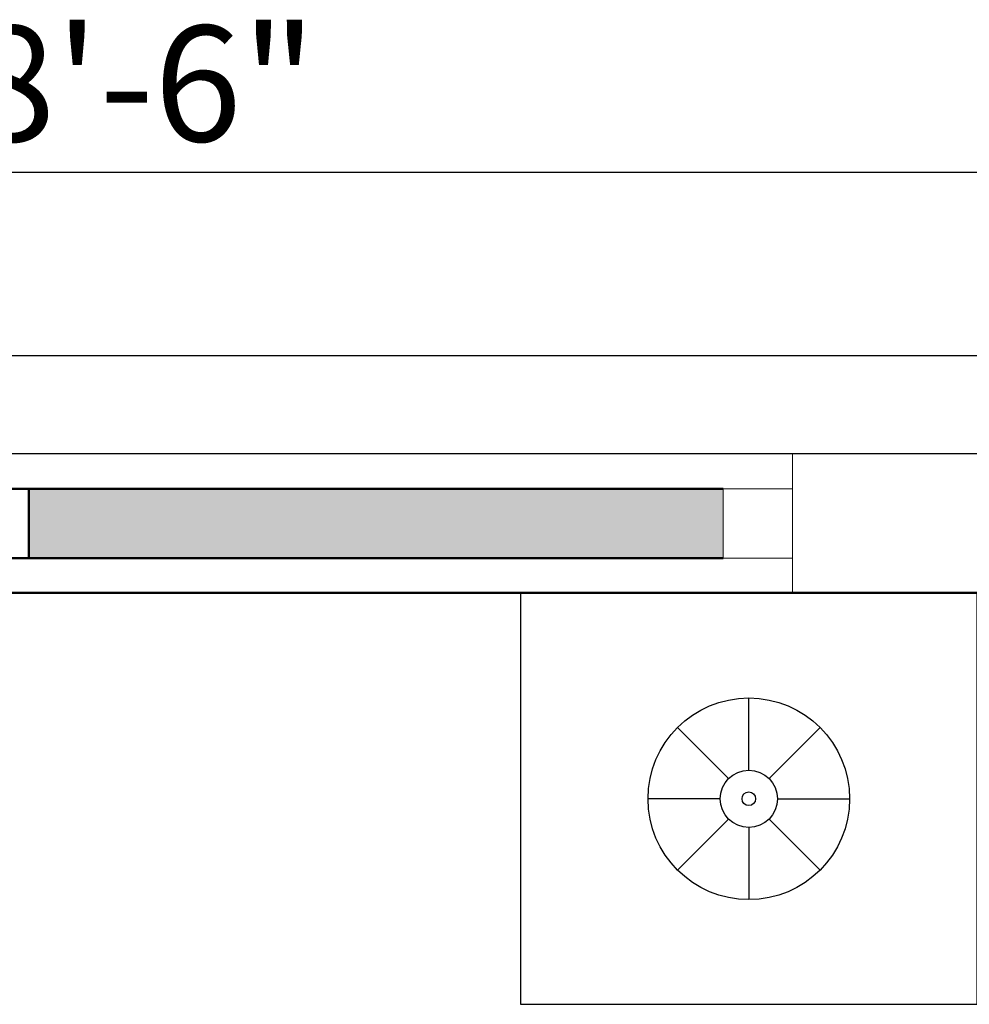
# Model space of a CAD drawing. Units: inches. Extents: x 3064 to 19385, y 846 to 15425.
# Tile 60 of 108: x 6210 to 6251, y 1964 to 2007. Entities that reach past the tile are written whole.
import ezdxf

# ---------------------------------------------------------------- set-up
doc = ezdxf.new("R2010")
doc.units = ezdxf.units.IN
for name, color, linetype, lineweight in [('A-ANNO-DIMS', 2, 'Continuous', 18), ('A-FLOR-FIXT', 9, 'Continuous', 18), ('A-GLAZ', 4, 'Continuous', 18), ('A-WALL', 7, 'Continuous', 50), ('C-PROP', 6, 'Continuous', 25)]:
    doc.layers.add(name, color=color, linetype=linetype, lineweight=lineweight)
doc.layers.add('BLOCK', color=6, linetype='Continuous')
doc.styles.get("Standard").update_dxf_attribs({"font": 'arial.ttf'})
doc.dimstyles.new('ISO-25', dxfattribs={"dimtxt": 9, "dimasz": 2.5, "dimexe": 1.25, "dimexo": 0.625, "dimtad": 1, "dimdec": 1, "dimlunit": 3, "dimtxsty": 'Standard', "dimcen": 2.5, "dimadec": 0, "dimazin": 0, "dimtfac": 1, "dimtdec": 1, "dimtmove": 0, "dimatfit": 3, "dimfxl": 1, "dimarcsym": 0})

# ---------------------------------------------------------------- blocks, each defined once
blk = doc.blocks.new('A$C52E67D0D')
at = {"layer": 'BLOCK'}
for p, q in [((250.5, 1605.5), (250.5, 1684.7)), ((228.3, 1596.3), (172.3, 1652.3)), ((272.7, 1596.3), (328.7, 1652.3)), ((219.1, 1574.1), (139.9, 1574.1)), ((281.9, 1574.1), (361.1, 1574.1)), ((228.3, 1551.9), (172.3, 1495.9)), ((272.7, 1551.9), (328.7, 1495.9)), ((250.5, 1542.8), (250.5, 1463.5))]:
    blk.add_line(p, q, dxfattribs=at)
blk.add_lwpolyline([(501, 1348.6), (501, 1799.6), (0, 1799.6), (0, 1348.6)], close=True, dxfattribs=at)
for radius in [110.6, 31.4, 7.46]:
    blk.add_circle((250.5, 1574.1), radius, dxfattribs=at)
blk = doc.blocks.new('*D387')
at = {"layer": 'A-ANNO-DIMS', "color": 0, "lineweight": -2, "transparency": 16777216}
for p, q in [((6183.493, 1988.614), (6183.493, 1993.494)), ((6378.493, 1988.614), (6378.493, 1993.494)), ((6185.993, 1992.244), (6375.993, 1992.244))]:
    blk.add_line(p, q, dxfattribs=at)
at = {"layer": 'A-ANNO-DIMS', "color": 0, "transparency": 16777216}
for points in [[(6185.993, 1992.66), (6185.993, 1991.827), (6183.493, 1992.244)], [(6375.993, 1992.66), (6375.993, 1991.827), (6378.493, 1992.244)]]:
    blk.add_solid(points, dxfattribs=at)
at = {"layer": 'Defpoints', "color": 0, "transparency": 16777216}
for p in [(6378.493, 1992.244), (6183.493, 1987.989), (6378.493, 1987.989)]:
    blk.add_point(p, dxfattribs=at)
at = {"layer": 'A-ANNO-DIMS', "color": 0, "transparency": 16777216, "insert": (6280.993, 1995.423), "char_height": 5, "attachment_point": 5}
blk.add_mtext('16\'-3"', dxfattribs=at)
blk = doc.blocks.new('*D378')
at = {"layer": 'A-ANNO-DIMS', "color": 0, "lineweight": -2, "transparency": 16777216}
for p, q in [((6042.493, 1988.614), (6042.493, 2001.412)), ((6384.493, 1988.614), (6384.493, 2001.412)), ((6044.993, 2000.162), (6381.993, 2000.162))]:
    blk.add_line(p, q, dxfattribs=at)
at = {"layer": 'A-ANNO-DIMS', "color": 0, "transparency": 16777216}
for points in [[(6044.993, 2000.578), (6044.993, 1999.745), (6042.493, 2000.162)], [(6381.993, 2000.578), (6381.993, 1999.745), (6384.493, 2000.162)]]:
    blk.add_solid(points, dxfattribs=at)
at = {"layer": 'Defpoints', "color": 0, "transparency": 16777216}
for p in [(6384.493, 2000.162), (6042.493, 1987.989), (6384.493, 1987.989)]:
    blk.add_point(p, dxfattribs=at)
at = {"layer": 'A-ANNO-DIMS', "color": 0, "transparency": 16777216, "insert": (6213.493, 2003.34), "char_height": 5, "attachment_point": 5}
blk.add_mtext('28\'-6"', dxfattribs=at)

msp = doc.modelspace()

# ---------------------------------------------------------------- hatches: boundary and pattern name
at = {"layer": 'A-GLAZ'}
h = msp.add_hatch(color=256, dxfattribs=at)
h.dxf.hatch_style = 1
h.paths.add_polyline_path([(6240.493, 1986.489), (6210.493, 1986.489), (6210.493, 1983.489), (6240.493, 1983.489)])

# ---------------------------------------------------------------- linework, layer by layer
msp.add_line((6243.493, 1987.989), (6243.493, 1981.989), dxfattribs=at)
msp.add_lwpolyline([(6243.493, 1983.489), (6240.493, 1983.489), (6240.493, 1986.489), (6243.493, 1986.489)], close=True, dxfattribs=at)
at = {"layer": 'A-WALL'}
for p, q in [((6210.493, 1986.489), (6240.493, 1986.489)), ((6210.493, 1983.489), (6240.493, 1983.489)), ((6378.493, 1981.989), (6183.493, 1981.989))]:
    msp.add_line(p, q, dxfattribs=at)
msp.add_lwpolyline([(6210.493, 1983.489), (6207.493, 1983.489), (6207.493, 1986.489), (6210.493, 1986.489)], close=True, dxfattribs=at)
at = {"layer": 'C-PROP'}
msp.add_line((6384.493, 1987.989), (6042.493, 1987.989), dxfattribs=at)

# ---------------------------------------------------------------- block references
at = {"layer": 'A-FLOR-FIXT', "xscale": 0.039370099999992, "yscale": 0.039370099999992, "zscale": 0.039370099999992}
msp.add_blockref('A$C52E67D0D', (6231.741, 1911.123), dxfattribs=at)

# ---------------------------------------------------------------- dimensions: what is measured, and where the dimension line sits
at = {"layer": 'A-ANNO-DIMS'}
for base, p1, p2, override, picture, middle in [((6384.493, 2000.162), (6042.493, 1987.989), (6384.493, 1987.989), {"dimtxt": 5, "dimclrd": 0, "dimclre": 0, "dimclrt": 0}, '*D378', (6213.493, 2003.34)), ((6378.493, 1992.244), (6183.493, 1987.989), (6378.493, 1987.989), {"dimtxt": 5, "dimclrd": 0, "dimclre": 0, "dimclrt": 0, "dimtmove": 1}, '*D387', (6280.993, 1995.423))]:
    dim = msp.add_linear_dim(base=base, p1=p1, p2=p2, dimstyle='ISO-25', override=override, dxfattribs=at)
    dim.commit()
    dim.dimension.update_dxf_attribs({"geometry": picture, "text_midpoint": middle})

doc.saveas('drawing.dxf')
